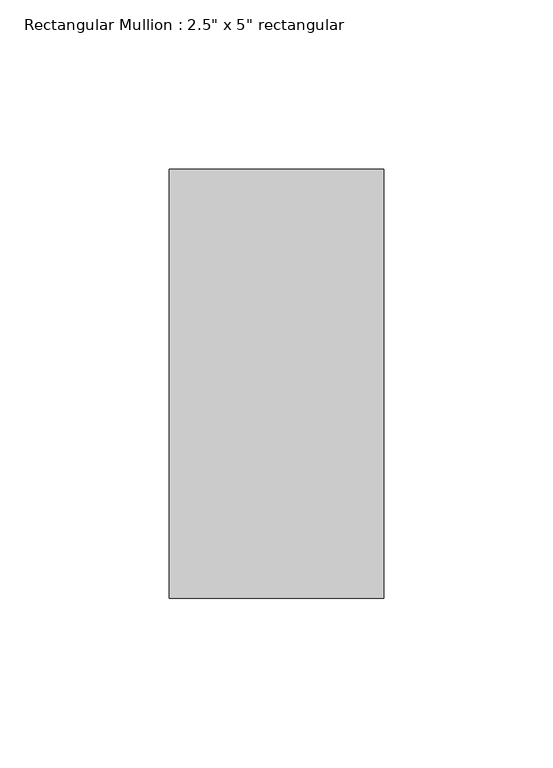
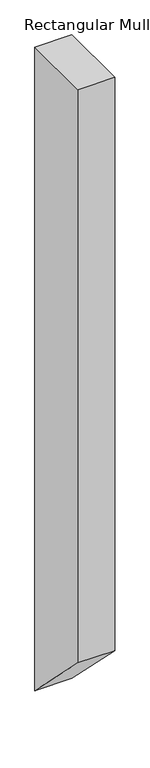
"""IFC4 building model written with IfcOpenShell, lengths in millimetres: member geometry."""

from ifc_helpers import new_model, si_unit, frame, origin, place, context, project, spatial, polyline, outline, extrude, source, transform, mapped, element, save


def member_637f24d3(model_context):
    return source(origin(), model_context, "Body", "SweptSolid", [
        extrude(outline(polyline([(-63.5, 0.0), (63.5, 0.0), (63.5, -1165.469231), (-63.5, -1038.469231), (-63.5, 0.0)])), frame((-31.75, 0.0, 0.0), z_axis=(1.0, 0.0, 0.0), x_axis=(0.0, 1.0, 0.0)), (0.0, 0.0, 1.0), 63.5),
    ])


if __name__ == "__main__":
    model = new_model("IFC4")
    model_context = context("Model", 3, world=origin())
    ifc_project = project(units=[si_unit("LENGTHUNIT", "METRE", prefix="MILLI")], contexts=[model_context])
    site = spatial("IfcSite", under=ifc_project)
    building = spatial("IfcBuilding", under=site)
    placement = place(None, origin())
    member_shape = member_637f24d3(model_context)
    element("IfcMember", 1, ObjectType="Rectangular Mullion : 2.5\" x 5\" rectangular", at=placement, inside=building, context=model_context, shape_type="MappedRepresentation", body=[
        mapped(member_shape, transform((0.0, 0.0, 0.0), x_axis=(1.0, 0.0, 0.0), y_axis=(0.0, 1.0, 0.0), z_axis=(0.0, 0.0, 1.0))),
    ])
    save(model, "model.ifc")

# Revit data of these elements
# Type "Rectangular Mullion : 2.5\" x 5\" rectangular"
#   built-in parameter 1007304 = 0.416667 (stored number, unit not read)
#   built-in parameter 1007301 = 0.104167 (stored number, unit not read)
#   built-in parameter 1007300 = 0.104167 (stored number, unit not read)
# Element 1 (IfcMember, "Rectangular Mullion : 2.5\" x 5\" rectangular")
#   Materials on its faces: "Aluminum"
# Materials
#   "Aluminum": class "Metal", colour RGB 247 247 247, transparency 0, Description = "Aluminum 6061", Cost = 0
